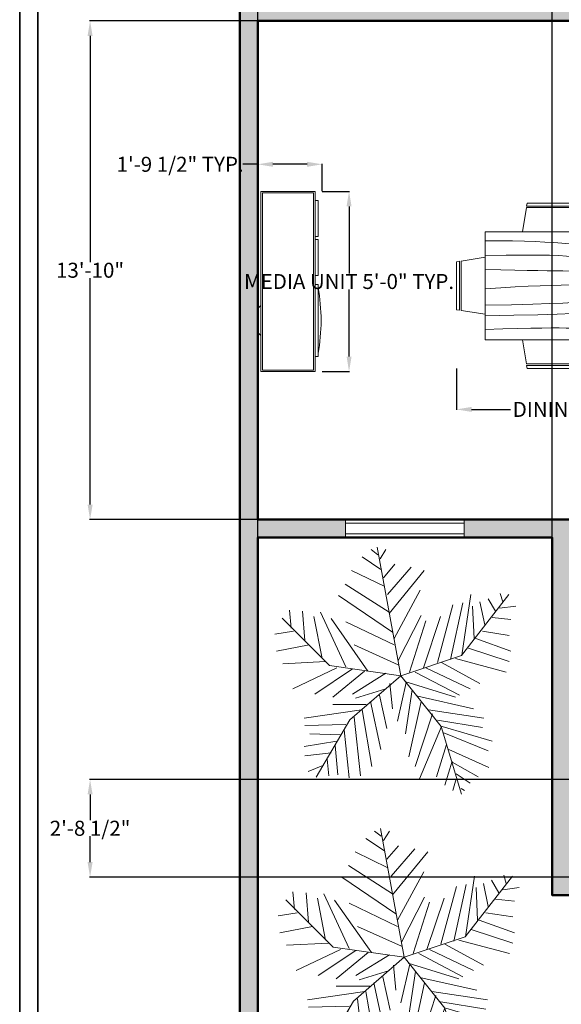
# Model space of a CAD drawing. Units: inches. Extents: x -60 to 743, y -483 to 510.
# Tile 2 of 7: x -60 to 120, y -299 to 29. Entities that reach past the tile are written whole.
import ezdxf

# ---------------------------------------------------------------- set-up
doc = ezdxf.new("R2010")
doc.units = ezdxf.units.IN
doc.header["$MEASUREMENT"] = 0
for name, color, linetype, lineweight in [('A-ANNO-DIMS', 2, 'Continuous', 18), ('A-ANNO-TTLB', 7, 'Continuous', 35), ('A-WALL-PATT', 30, 'Continuous', 13), ('FURNITURE', 40, 'Continuous', 18), ('TREES', 80, 'Continuous', 13), ('WALL BOUNDRY', 10, 'Continuous', 50), ('WINDOW', 200, 'Continuous', 18)]:
    doc.layers.add(name, color=color, linetype=linetype, lineweight=lineweight)
doc.styles.get("Standard").update_dxf_attribs({"font": 'arial.ttf'})
doc.dimstyles.get("Standard").update_dxf_attribs({"dimtxt": 5, "dimasz": 5, "dimexe": 0.18, "dimexo": 0.0625, "dimgap": 0.09, "dimtad": 0, "dimtih": 1, "dimtoh": 1, "dimdec": 1, "dimzin": 0, "dimdsep": 46, "dimlunit": 4, "dimtxsty": 'Standard', "dimcen": 0.09, "dimadec": 0, "dimazin": 0, "dimtfac": 1, "dimtdec": 1, "dimtofl": 0, "dimtmove": 0, "dimatfit": 3, "dimfxl": 1, "dimtolj": 1, "dimtzin": 0, "dimarcsym": 0})

# ---------------------------------------------------------------- blocks, each defined once
blk = doc.blocks.new('Dining Set - 36 x 72 in.')
for p, q in [((-22, 27.5), (-22.1562, 26.50042)), ((-5.8416, 26.5), (-22.1534, 26.5)), ((-22, 27.5), (-6, 27.5)), ((-5.8437, 26.49966), (-6, 27.5)), ((6, 27.5), (5.8438, 26.50042)), ((22.1584, 26.5), (5.8466, 26.5)), ((6, 27.5), (22, 27.5)), ((22.1563, 26.49966), (22, 27.5)), ((-22.2343, 26.00059), (-23.4847, 17.99762)), ((-22.2304, 26), (-5.7608, 26)), ((-4.5152, 17.99762), (-5.7655, 25.99926)), ((5.7657, 26.00059), (4.5153, 17.99762)), ((5.7696, 26), (22.2392, 26)), ((23.4848, 17.99762), (22.2345, 25.99926)), ((36, 18), (-36, 18)), ((-36, 18), (-36, -18)), ((36, -18), (36, 18)), ((-45.5, 8), (-44.5004, 8.15617)), ((-45.5, 8), (-45.5, -8)), ((-44.5, -8.15843), (-44.5, 8.15338)), ((-44.0006, 8.23428), (-35.9976, 9.48474)), ((-44, 8.23041), (-44, -8.23915)), ((44.0006, 8.23428), (35.9976, 9.48474)), ((44, 8.23041), (44, -8.23915)), ((44.5, -8.15843), (44.5, 8.15338)), ((45.5, 8), (44.5005, 8.15617)), ((45.5, 8), (45.5, -8)), ((-44.4997, -8.15631), (-45.5, -8)), ((-35.9976, -9.48476), (-43.9993, -8.2345)), ((35.9976, -9.48476), (43.9993, -8.2345)), ((44.4997, -8.15631), (45.5, -8)), ((-36, -18), (36, -18)), ((-22.2343, -26.0006), (-23.4847, -17.99762)), ((-4.5152, -17.99762), (-5.7655, -25.99928)), ((5.7657, -26.0006), (4.5153, -17.99762)), ((23.4848, -17.99762), (22.2345, -25.99928)), ((-22.2304, -26), (-5.7608, -26)), ((5.7696, -26), (22.2392, -26)), ((-22, -27.5), (-22.1562, -26.50044)), ((-5.8416, -26.5), (-22.1534, -26.5)), ((-22, -27.5), (-6, -27.5)), ((-5.8437, -26.49967), (-6, -27.5)), ((6, -27.5), (5.8438, -26.50044)), ((22.1584, -26.5), (5.8466, -26.5)), ((6, -27.5), (22, -27.5)), ((22.1563, -26.49967), (22, -27.5))]:
    blk.add_line(p, q)
for points in [[(-36, 15), (-31.1772, 14.97754), (-26.8079, 14.91406), (-22.8538, 14.81543), (-19.276, 14.6875), (-16.0362, 14.53613), (-13.0957, 14.36718), (-10.4159, 14.18652), (-7.9583, 14), (-5.6904, 13.81315), (-3.6035, 13.63021), (-1.6954, 13.45508), (0.0365, 13.29166), (1.5945, 13.14388), (2.9811, 13.01562), (4.1988, 12.9108), (5.25, 12.83333), (6.1393, 12.78613), (6.8802, 12.76823), (7.4883, 12.77767), (7.9792, 12.8125), (8.3685, 12.87077), (8.6719, 12.95052), (8.9049, 13.0498), (9.0833, 13.16666), (9.2205, 13.29899), (9.3216, 13.44401), (9.3895, 13.59879), (9.4271, 13.76041), (9.4373, 13.92594), (9.4232, 14.09245), (9.3875, 14.257), (9.3333, 14.41666), (9.2638, 14.56917), (9.1836, 14.71484), (9.0975, 14.85465), (9.0104, 14.98958), (8.9272, 15.1206), (8.8529, 15.2487), (8.7922, 15.37483), (8.75, 15.5), (8.7305, 15.62467), (8.7344, 15.74739), (8.7617, 15.86621), (8.8125, 15.97916), (8.8867, 16.08431), (8.9844, 16.17968), (9.1055, 16.26334), (9.25, 16.33333), (9.4189, 16.38802), (9.6172, 16.42708), (9.8506, 16.45052), (10.125, 16.45833), (10.4463, 16.45052), (10.8203, 16.42708), (11.2529, 16.38802), (11.75, 16.33333), (12.3184, 16.26318), (12.9694, 16.17838), (13.7151, 16.07991), (14.5677, 15.96875), (15.5395, 15.84586), (16.6426, 15.71224), (17.8893, 15.56884), (19.2917, 15.41666), (20.859, 15.25667), (22.5879, 15.08984), (24.4721, 14.91715), (26.5052, 14.73958), (28.6809, 14.5581), (30.9929, 14.3737), (33.4347, 14.18733), (36, 14)], [(-36, 10), (-28.9766, 10.14274), (-23.1725, 10.20442), (-18.4241, 10.19775), (-14.5677, 10.13541), (-11.4399, 10.03011), (-8.877, 9.89453), (-6.7154, 9.74137), (-4.7917, 9.58333), (-2.9698, 9.43082), (-1.2246, 9.28515), (0.4415, 9.14534), (2.026, 9.01041), (3.5266, 8.87939), (4.9408, 8.7513), (6.266, 8.62516), (7.5, 8.5), (8.6411, 8.37549), (9.6914, 8.2539), (10.6538, 8.13818), (11.5312, 8.03125), (12.3267, 7.93603), (13.043, 7.85547), (13.6831, 7.79248), (14.25, 7.75), (14.7471, 7.7303), (15.1797, 7.73307), (15.5537, 7.75732), (15.875, 7.80208), (16.1494, 7.86637), (16.3828, 7.94922), (16.5811, 8.04964), (16.75, 8.16666), (16.8944, 8.29915), (17.0143, 8.44531), (17.1089, 8.60319), (17.1771, 8.77083), (17.218, 8.94629), (17.2305, 9.1276), (17.2137, 9.31282), (17.1667, 9.5), (17.0895, 9.6875), (16.987, 9.875), (16.8649, 10.0625), (16.7292, 10.25), (16.5856, 10.4375), (16.4401, 10.625), (16.2985, 10.8125), (16.1667, 11), (16.05, 11.18733), (15.9518, 11.3737), (15.8752, 11.5581), (15.8229, 11.73958), (15.798, 11.91715), (15.8034, 12.08984), (15.842, 12.25667), (15.9167, 12.41666), (16.0295, 12.56836), (16.1784, 12.70833), (16.3605, 12.83268), (16.5729, 12.9375), (16.8127, 13.01888), (17.0768, 13.07291), (17.3625, 13.0957), (17.6667, 13.08333), (17.9894, 13.03312), (18.3418, 12.94726), (18.7382, 12.82918), (19.1927, 12.68229), (19.7195, 12.51001), (20.3327, 12.31575), (21.0465, 12.10294), (21.875, 11.875), (22.8357, 11.63354), (23.959, 11.37304), (25.2786, 11.08618), (26.8282, 10.76562), (28.6414, 10.40405), (30.752, 9.99414), (33.1936, 9.52856), (36, 9)], [(-36, 5.5), (-30.7157, 5.3348), (-26.069, 5.20963), (-21.9946, 5.11767), (-18.4271, 5.05208), (-15.3009, 5.00602), (-12.5508, 4.97265), (-10.1112, 4.94515), (-7.9167, 4.91666), (-5.909, 4.88167), (-4.0586, 4.83984), (-2.3429, 4.79215), (-0.7396, 4.73958), (0.7739, 4.6831), (2.22, 4.6237), (3.6213, 4.56233), (5, 4.5), (6.373, 4.43782), (7.7344, 4.3776), (9.0723, 4.32129), (10.375, 4.27083), (11.6309, 4.22819), (12.8281, 4.19531), (13.9551, 4.17415), (15, 4.16666), (15.954, 4.17448), (16.819, 4.19791), (17.6001, 4.23698), (18.3021, 4.29166), (18.9299, 4.36198), (19.4883, 4.44791), (19.9823, 4.54948), (20.4167, 4.66666), (20.7969, 4.79899), (21.1302, 4.94401), (21.4245, 5.09879), (21.6875, 5.26041), (21.9271, 5.42594), (22.1511, 5.59245), (22.3672, 5.757), (22.5834, 5.91666), (22.8065, 6.06868), (23.0404, 6.21093), (23.2879, 6.34147), (23.5521, 6.45833), (23.8358, 6.55957), (24.142, 6.64323), (24.4735, 6.70735), (24.8334, 6.75), (25.2235, 6.76969), (25.642, 6.76692), (26.0858, 6.74267), (26.5521, 6.69791), (27.0379, 6.63362), (27.5404, 6.55078), (28.0565, 6.45036), (28.5834, 6.33333), (29.1242, 6.19987), (29.7071, 6.04687), (30.3661, 5.87044), (31.1354, 5.66666), (32.0493, 5.43164), (33.142, 5.16146), (34.4475, 4.85221), (36, 4.5)], [(-36, -1), (-30.7915, -0.6591), (-26.0195, -0.38216), (-21.6519, -0.16284), (-17.6563, 0.00521), (-14.0005, 0.12833), (-10.6523, 0.21289), (-7.5796, 0.26522), (-4.75, 0.29166), (-2.134, 0.29793), (0.2878, 0.28711), (2.5317, 0.26163), (4.6146, 0.22396), (6.5529, 0.17651), (8.3633, 0.12174), (10.0623, 0.06209), (11.6667, 0), (13.1899, -0.06201), (14.6341, -0.1211), (15.9982, -0.17432), (17.2813, -0.21875), (18.4823, -0.25147), (19.6003, -0.26953), (20.6343, -0.27002), (21.5834, -0.25), (22.4481, -0.20768), (23.2357, -0.14584), (23.9549, -0.06836), (24.6146, 0.02083), (25.2235, 0.11784), (25.7904, 0.21875), (26.3241, 0.31966), (26.8334, 0.41666), (27.3265, 0.50618), (27.8099, 0.58593), (28.2894, 0.65397), (28.7709, 0.70833), (29.2601, 0.74707), (29.763, 0.76823), (30.2855, 0.76985), (30.8334, 0.75), (31.4088, 0.70784), (31.9994, 0.64713), (32.589, 0.57275), (33.1615, 0.48958), (33.7008, 0.4025), (34.1908, 0.3164), (34.6153, 0.23616), (34.9584, 0.16666), (35.2099, 0.11165), (35.3848, 0.07031), (35.504, 0.04069), (35.5886, 0.02083), (35.6594, 0.00879), (35.7377, 0.0026), (35.8442, 0.00032), (36, 0)], [(-36, -6.5), (-27.1843, -6.31267), (-20.084, -6.1263), (-14.469, -5.9419), (-10.1094, -5.76042), (-6.7752, -5.58285), (-4.2363, -5.41016), (-2.2629, -5.24333), (-0.625, -5.08334), (0.8708, -4.93099), (2.2715, -4.78646), (3.5872, -4.64974), (4.8281, -4.52084), (6.0046, -4.39974), (7.127, -4.28646), (8.2053, -4.18099), (9.25, -4.08334), (10.2705, -3.99382), (11.2734, -3.91407), (12.2647, -3.84603), (13.25, -3.79167), (14.2354, -3.75293), (15.2266, -3.73177), (16.2295, -3.73015), (17.25, -3.75), (18.2912, -3.79248), (19.3451, -3.85547), (20.4009, -3.93604), (21.4479, -4.03125), (22.4754, -4.13819), (23.4727, -4.25391), (24.4289, -4.37549), (25.3334, -4.5), (26.1785, -4.62492), (26.9694, -4.74935), (27.7145, -4.87281), (28.4219, -4.99479), (29.1, -5.11483), (29.7572, -5.23242), (30.4016, -5.34709), (31.0417, -5.45834), (31.6837, -5.56437), (32.3262, -5.65821), (32.9658, -5.73153), (33.599, -5.77604), (34.2224, -5.78345), (34.8327, -5.74545), (35.4264, -5.65373), (36, -5.5)], [(-36, -10), (-26.4022, -9.81299), (-18.4675, -9.62891), (-11.9839, -9.45069), (-6.7396, -9.28125), (-2.5226, -9.12354), (0.8789, -8.98047), (3.6769, -8.85498), (6.0833, -8.75), (8.2767, -8.66765), (10.3021, -8.60677), (12.1712, -8.56543), (13.8958, -8.54167), (15.4876, -8.53353), (16.9583, -8.53907), (18.3197, -8.55632), (19.5834, -8.58334), (20.7616, -8.61841), (21.8685, -8.66081), (22.9188, -8.71004), (23.9271, -8.76563), (24.9081, -8.82707), (25.8763, -8.89388), (26.8465, -8.96558), (27.8334, -9.04167), (28.8474, -9.12118), (29.8828, -9.20117), (30.93, -9.27824), (31.9792, -9.34896), (33.0205, -9.40991), (34.0443, -9.45768), (35.0407, -9.48885), (36, -9.5)], [(-36, -14.5), (-30.0881, -14.33513), (-25.0332, -14.21224), (-20.7312, -14.12647), (-17.0781, -14.07292), (-13.97, -14.04671), (-11.3027, -14.04297), (-8.9724, -14.05681), (-6.875, -14.08334), (-4.9224, -14.11833), (-3.0905, -14.16016), (-1.3709, -14.20785), (0.2448, -14.26042), (1.7647, -14.3169), (3.1973, -14.3763), (4.5507, -14.43767), (5.8333, -14.5), (7.0554, -14.5621), (8.235, -14.62175), (9.3922, -14.67652), (10.5469, -14.72396), (11.7192, -14.76164), (12.929, -14.78711), (14.1965, -14.79794), (15.5417, -14.79167), (16.9933, -14.76424), (18.6152, -14.70508), (20.4804, -14.60197), (22.6615, -14.44271), (25.2312, -14.21509), (28.2624, -13.9069), (31.8277, -13.50594), (36, -13)]]:
    blk.add_lwpolyline(points)
blk = doc.blocks.new('Entertainment Center')
for p, q in [((-4, 0), (-5, -1)), ((4, 0), (-4, 0)), ((5, -1), (4, 0)), ((-17, -19), (-17, -1)), ((-17, -1), (43, -1)), ((-16.5, -18.5), (-16.5, -1.5)), ((-16.5, -1.5), (42.5, -1.5)), ((42.5, -1.5), (42.5, -18.5)), ((43, -1), (43, -19)), ((43, -19), (-17, -19)), ((42.5, -18.5), (-16.5, -18.5)), ((-12, -20), (-12, -19)), ((12, -19), (12, -20)), ((15, -20), (15, -19)), ((27, -19), (27, -20)), ((28, -20), (28, -19)), ((40, -19), (40, -20)), ((12, -20), (-12, -20)), ((27, -20), (15, -20)), ((40, -20), (28, -20))]:
    blk.add_line(p, q)
blk.add_arc((0, 40), 61, 259.6111, 280.3889)
blk = doc.blocks.new('*U21')
for p, q in [((0, 0), (-266.7, 1447.8)), ((-221.9198, 1197.3052), (-433.5526, 1338.8594)), ((-258.7244, 1362.456), (-332.3336, 1421.4348)), ((-231.1146, 1315.2628), (-166.7002, 1421.4348)), ((-194.31, 1102.9442), (-65.4812, 1256.284)), ((-148.3106, 914.1968), (118.5418, 1220.9018)), ((-185.1152, 1008.5578), (-553.1612, 1185.4942)), ((-129.8956, 701.8528), (265.7602, 1185.4942)), ((-129.8956, 713.6638), (-626.7704, 1032.1544)), ((-93.091, 489.5342), (-700.3796, 902.3858)), ((-74.7014, 418.7444), (219.7608, 961.39)), ((685.8, 228.6), (1219.2, 914.4)), ((689.0258, 230.0224), (790.2448, 914.1968)), ((1121.4862, 925.9824), (1149.0706, 831.6214)), ((412.9786, 147.447), (587.8068, 796.2392)), ((560.197, 182.8292), (698.2206, 819.8358)), ((808.6344, 784.4282), (827.0494, 418.7444)), ((891.4384, 831.6214), (946.658, 572.1096)), ((983.4626, 867.0036), (1066.2666, 725.4494)), ((1112.2914, 760.8316), (1296.3144, 784.4282)), ((-1234.059, 536.7274), (-1252.4486, 737.2604)), ((-1105.2302, 725.4494), (-1077.6458, 395.1732)), ((-976.4268, 666.4706), (-884.4026, 194.6402)), ((-902.8176, 713.6638), (-617.5756, 100.2538)), ((-28.6766, 171.0436), (228.9556, 678.2816)), ((256.5654, 88.4682), (449.7832, 666.4706)), ((-800.1, 114.3), (-1333.5, 647.7)), ((-369.1382, 53.086), (-783.1836, 642.874)), ((-617.5756, 607.4918), (-74.7014, 347.98)), ((100.1268, 41.275), (284.1498, 619.2774)), ((1029.462, 654.685), (1241.0948, 631.0884)), ((-1206.4492, 501.3198), (-1418.082, 465.9376)), ((919.0482, 501.3198), (1222.6798, 454.152)), ((-1031.621, 347.98), (-1399.667, 277.1902)), ((-525.5514, 347.98), (-28.6766, 123.8504)), ((845.439, 418.7444), (1241.0948, 277.1902)), ((0, 0), (685.8, 228.6)), ((753.4148, 312.5978), (1222.6798, 159.2326)), ((-847.598, 159.2326), (-1326.0578, 135.636)), ((0, 0), (-800.1, 114.3)), ((458.978, 147.447), (891.4384, -88.4682)), ((615.4166, 194.6402), (1185.8752, 41.275)), ((-718.7946, 88.4682), (-1215.644, -147.447)), ((-543.9664, 76.6572), (-967.2066, -206.4512)), ((-405.9428, 53.086), (-764.794, -241.8334)), ((0, 0), (-571.5, -495.3)), ((-166.7002, 29.4894), (-543.9664, -206.4512)), ((0, 0), (457.2, -571.5)), ((164.5412, 41.275), (661.416, -218.2368)), ((284.1498, 88.4682), (781.0246, -147.447)), ((-120.7008, -88.4682), (-93.091, -371.5766)), ((63.3222, -76.6826), (-37.8714, -513.1308)), ((44.9326, -64.897), (615.4166, -241.8334)), ((-166.7002, -147.447), (-507.1618, -253.619)), ((-240.3094, -218.2368), (-157.5054, -595.7062)), ((127.7366, -159.258), (54.1274, -654.685)), ((-387.5278, -324.4088), (-764.794, -324.4088)), ((-341.5284, -289.0012), (-221.9198, -831.6214)), ((228.9556, -289.0012), (90.932, -914.1968)), ((192.151, -230.0224), (817.8292, -371.5766)), ((-442.7474, -383.3876), (-1086.8406, -477.7486)), ((-433.5526, -383.3876), (-323.1134, -1020.3688)), ((357.759, -430.5554), (164.5412, -1020.3688)), ((311.7596, -383.3876), (937.4378, -477.7486)), ((-617.5756, -548.5384), (-1077.6458, -560.324)), ((-571.5, -495.3), (-952.5, -1143)), ((-525.5514, -465.963), (-451.9422, -1126.5408)), ((412.9786, -501.3452), (919.0482, -583.9206)), ((-681.9646, -666.496), (-1022.4262, -654.685)), ((-635.9652, -607.5172), (-580.771, -1150.1374)), ((458.978, -572.1096), (210.5406, -1161.923)), ((457.2, -571.5), (685.8, -1333.5)), ((468.1982, -572.1096), (1029.462, -737.2604)), ((486.5878, -642.8994), (983.4626, -843.4324)), ((-718.7946, -737.2604), (-1086.8406, -796.2392)), ((514.1976, -772.6426), (403.7838, -1138.3264)), ((-783.1836, -867.029), (-1077.6458, -902.4112)), ((-737.1842, -784.4536), (-709.5744, -1114.7298)), ((541.8074, -831.6214), (992.6574, -1032.1544)), ((-829.2084, -937.7934), (-810.7934, -1126.5408)), ((578.612, -961.39), (495.7826, -1232.7128)), ((578.612, -973.1756), (873.0488, -1138.3264)), ((-875.2078, -1008.5832), (-1040.8412, -1079.3476)), ((624.6114, -1102.9442), (781.0246, -1209.1162)), ((624.6114, -1161.923), (587.8068, -1291.6916)), ((679.8056, -1268.095), (716.6102, -1291.6916))]:
    blk.add_line(p, q)
blk = doc.blocks.new('*D36')
at = {"layer": 'A-ANNO-DIMS', "color": 0, "lineweight": -2, "transparency": 16777216}
for p, q in [((40.54, -28.32), (49.66, -28.32)), ((49.48, -33.32), (49.48, -55.67)), ((49.48, -83.32), (49.48, -60.96)), ((40.54, -88.32), (49.66, -88.32))]:
    blk.add_line(p, q, dxfattribs=at)
at = {"layer": 'A-ANNO-DIMS', "color": 0, "transparency": 16777216}
for points in [[(48.65, -33.32), (50.31, -33.32), (49.48, -28.32)], [(48.65, -83.32), (50.31, -83.32), (49.48, -88.32)]]:
    blk.add_solid(points, dxfattribs=at)
at = {"layer": 'Defpoints', "color": 0, "transparency": 16777216}
for p in [(40.48, -28.32), (49.48, -28.32), (40.48, -88.32)]:
    blk.add_point(p, dxfattribs=at)
at = {"layer": 'A-ANNO-DIMS', "color": 0, "transparency": 16777216, "insert": (49.48, -58.32), "char_height": 5, "attachment_point": 5}
blk.add_mtext('\\A1;MEDIA UNIT 5\'-0" TYP.', dxfattribs=at)
blk = doc.blocks.new('*D37')
at = {"layer": 'A-ANNO-DIMS', "color": 0, "lineweight": -2, "transparency": 16777216}
for p, q in [((19.15, -19.32), (14.15, -19.32)), ((19.15, -28.25), (19.15, -19.14)), ((35.48, -19.32), (24.15, -19.32)), ((40.48, -28.25), (40.48, -19.14))]:
    blk.add_line(p, q, dxfattribs=at)
at = {"layer": 'A-ANNO-DIMS', "color": 0, "transparency": 16777216}
for points in [[(24.15, -18.48), (24.15, -20.15), (19.15, -19.32)], [(35.48, -18.48), (35.48, -20.15), (40.48, -19.32)]]:
    blk.add_solid(points, dxfattribs=at)
at = {"layer": 'Defpoints', "color": 0, "transparency": 16777216}
for p in [(19.15, -19.32), (19.15, -28.32), (40.48, -28.32)]:
    blk.add_point(p, dxfattribs=at)
at = {"layer": 'A-ANNO-DIMS', "color": 0, "transparency": 16777216, "insert": (-6.77, -19.32), "char_height": 5, "attachment_point": 5}
blk.add_mtext('\\A1;1\'-9 1/2" TYP.', dxfattribs=at)
blk = doc.blocks.new('*D62')
at = {"layer": 'A-ANNO-DIMS', "color": 0, "lineweight": -2, "transparency": 16777216}
for p, q in [((85.25, -87.32), (85.25, -101.08)), ((176.25, -87.32), (176.25, -101.08)), ((90.25, -100.9), (103.18, -100.9)), ((171.25, -100.9), (158.32, -100.9))]:
    blk.add_line(p, q, dxfattribs=at)
at = {"layer": 'A-ANNO-DIMS', "color": 0, "transparency": 16777216}
for points in [[(90.25, -100.07), (90.25, -101.74), (85.25, -100.9)], [(171.25, -100.07), (171.25, -101.74), (176.25, -100.9)]]:
    blk.add_solid(points, dxfattribs=at)
at = {"layer": 'Defpoints', "color": 0, "transparency": 16777216}
for p in [(85.25, -87.25), (176.25, -87.25), (176.25, -100.9)]:
    blk.add_point(p, dxfattribs=at)
at = {"layer": 'A-ANNO-DIMS', "color": 0, "transparency": 16777216, "insert": (130.75, -100.9), "char_height": 5, "attachment_point": 5}
blk.add_mtext('\\A1;DINING SET 7\'-7"', dxfattribs=at)
blk = doc.blocks.new('*D72')
at = {"layer": 'A-ANNO-DIMS', "color": 0, "lineweight": -2, "transparency": 16777216}
for p, q in [((19.08, 28.42), (-36.93, 28.42)), ((-36.75, 23.42), (-36.75, -51.93)), ((-36.75, -132.58), (-36.75, -57.22)), ((19.08, -137.58), (-36.93, -137.58))]:
    blk.add_line(p, q, dxfattribs=at)
at = {"layer": 'A-ANNO-DIMS', "color": 0, "transparency": 16777216}
for points in [[(-37.58, 23.42), (-35.91, 23.42), (-36.75, 28.42)], [(-37.58, -132.58), (-35.91, -132.58), (-36.75, -137.58)]]:
    blk.add_solid(points, dxfattribs=at)
at = {"layer": 'Defpoints', "color": 0, "transparency": 16777216}
for p in [(19.15, 28.42), (-36.75, -137.58), (19.15, -137.58)]:
    blk.add_point(p, dxfattribs=at)
at = {"layer": 'A-ANNO-DIMS', "color": 0, "transparency": 16777216, "insert": (-36.75, -54.58), "char_height": 5, "attachment_point": 5}
blk.add_mtext('\\A1;13\'-10"', dxfattribs=at)
blk = doc.blocks.new('*D73')
at = {"layer": 'A-ANNO-DIMS', "color": 0, "lineweight": -2, "transparency": 16777216}
for p, q in [((19.15, -143.52), (19.15, 465.7)), ((24.15, 465.52), (61.41, 465.52)), ((112.15, 465.52), (74.89, 465.52)), ((117.15, -143.52), (117.15, 465.7))]:
    blk.add_line(p, q, dxfattribs=at)
at = {"layer": 'A-ANNO-DIMS', "color": 0, "transparency": 16777216}
for points in [[(24.15, 466.36), (24.15, 464.69), (19.15, 465.52)], [(112.15, 466.36), (112.15, 464.69), (117.15, 465.52)]]:
    blk.add_solid(points, dxfattribs=at)
at = {"layer": 'Defpoints', "color": 0, "transparency": 16777216}
for p in [(117.15, 465.52), (19.15, -143.58), (117.15, -143.58)]:
    blk.add_point(p, dxfattribs=at)
at = {"layer": 'A-ANNO-DIMS', "color": 0, "transparency": 16777216, "insert": (68.15, 465.52), "char_height": 5, "attachment_point": 5}
blk.add_mtext('\\A1;8\'-2"', dxfattribs=at)
blk = doc.blocks.new('*D77')
at = {"layer": 'A-ANNO-DIMS', "color": 0, "lineweight": -2, "transparency": 16777216}
for p, q in [((154.93, -224.05), (-36.93, -224.05)), ((-36.75, -229.05), (-36.75, -237.64)), ((-36.75, -251.58), (-36.75, -242.99)), ((123.08, -256.58), (-36.93, -256.58))]:
    blk.add_line(p, q, dxfattribs=at)
at = {"layer": 'A-ANNO-DIMS', "color": 0, "transparency": 16777216}
for points in [[(-37.58, -229.05), (-35.91, -229.05), (-36.75, -224.05)], [(-37.58, -251.58), (-35.91, -251.58), (-36.75, -256.58)]]:
    blk.add_solid(points, dxfattribs=at)
at = {"layer": 'Defpoints', "color": 0, "transparency": 16777216}
for p in [(154.99, -224.05), (-36.75, -256.58), (123.15, -256.58)]:
    blk.add_point(p, dxfattribs=at)
at = {"layer": 'A-ANNO-DIMS', "color": 0, "transparency": 16777216, "insert": (-36.75, -240.31), "char_height": 5, "attachment_point": 5}
blk.add_mtext('\\A1;2\'-8 1/2"', dxfattribs=at)

msp = doc.modelspace()

# ---------------------------------------------------------------- hatches: boundary and pattern name
at = {"layer": 'A-WALL-PATT'}
h = msp.add_hatch(color=256, dxfattribs=at)
h.dxf.hatch_style = 1
h.paths.add_polyline_path([(412.35, 168.77), (415.89, 168.77), (415.89, 114.92), (412.35, 114.92)], flags=16)
h.paths.add_polyline_path([(87.81, -138.81), (87.81, -142.35), (48.31, -142.32), (48.31, -138.78)], flags=16)
h.paths.add_polyline_path([(459.53, -138.78), (513.39, -138.78), (513.39, -142.32), (459.53, -142.32)], flags=16)
h.paths.add_polyline_path([(164.84, -257.78), (218.7, -257.78), (218.7, -261.32), (164.84, -261.32)], flags=16)
h.paths.add_polyline_path([(417.15, 114.92), (415.89, 114.92), (415.89, 168.77), (417.15, 168.77), (417.15, 195.42), (411.15, 195.42), (411.15, 168.77), (412.35, 168.77), (412.35, 114.92), (411.15, 114.92), (411.15, 28.42), (610.15, 28.42), (610.15, -43.58), (508.15, -43.58), (508.15, -49.58), (610.15, -49.58), (610.15, -137.58), (513.39, -137.58), (513.39, -138.78), (459.53, -138.78), (459.53, -137.58), (359.15, -137.58), (359.15, -143.58), (377.15, -143.58), (377.15, -292.58), (383.15, -292.58), (383.15, -143.58), (459.53, -143.58), (459.53, -142.32), (513.39, -142.32), (513.39, -143.58), (610.15, -143.58), (610.15, -415.58), (610.15, -421.58), (616.15, -421.58), (616.15, 418.42), (13.15, 418.42), (13.15, -421.58), (19.15, -421.58), (430.15, -421.58), (430.15, -415.58), (19.15, -415.58), (19.15, -143.58), (48.31, -143.58), (48.31, -142.32), (87.81, -142.35), (87.81, -143.58), (117.15, -143.58), (117.15, -262.58), (164.84, -262.58), (164.84, -261.32), (218.7, -261.32), (218.7, -262.58), (273.15, -262.58), (273.15, -292.58), (279.15, -292.58), (279.15, -143.58), (297.15, -143.58), (297.15, -137.58), (273.15, -137.58), (273.15, -256.58), (218.7, -256.58), (218.7, -257.78), (164.84, -257.78), (164.84, -256.58), (123.15, -256.58), (123.15, -143.58), (225.15, -143.58), (225.15, -137.58), (87.81, -137.58), (87.81, -138.81), (48.31, -138.78), (48.31, -137.58), (19.15, -137.58), (19.15, 28.42), (187.15, 28.42), (187.15, 34.42), (19.15, 34.42), (19.15, 178.42), (273.15, 178.42), (273.15, 184.42), (19.15, 184.42), (19.15, 345.58), (195.14, 345.58), (195.14, 348.9), (19.15, 348.9), (19.15, 412.42), (267.15, 412.42), (267.15, 319.83), (273.15, 319.83), (273.15, 412.42), (411.15, 412.42), (411.15, 376.24), (417.15, 376.24), (417.15, 412.42), (610.15, 412.42), (610.15, 249.42), (411.15, 249.42), (411.15, 243.42), (610.15, 243.42), (610.15, 34.42), (417.15, 34.42)])
h = msp.add_hatch(color=256, dxfattribs=at)
h.dxf.hatch_style = 1
h.paths.add_polyline_path([(273.15, 265.98), (267.15, 265.98), (267.15, 232.42), (273.15, 232.42)])
h.paths.add_polyline_path([(417.15, 322.39), (411.15, 322.39), (411.15, 297.42), (417.15, 297.42)])
h.paths.add_polyline_path([(417.15, 195.42), (411.15, 195.42), (411.15, 168.77), (417.15, 168.77)])
h.paths.add_polyline_path([(459.53, -137.58), (359.15, -137.58), (359.15, -143.58), (377.15, -143.58), (377.15, -292.58), (383.15, -292.58), (383.15, -143.58), (459.53, -143.58)])
h.paths.add_polyline_path([(279.15, -143.58), (297.15, -143.58), (297.15, -137.58), (273.15, -137.58), (273.15, -256.58), (218.7, -256.58), (218.7, -262.58), (273.15, -262.58), (273.15, -292.58), (279.15, -292.58)])
h.paths.add_polyline_path([(123.15, -143.58), (225.15, -143.58), (225.15, -137.58), (87.81, -137.58), (87.81, -143.58), (117.15, -143.58), (117.15, -262.58), (164.84, -262.58), (164.84, -256.58), (123.15, -256.58)])
h = msp.add_hatch(color=256, dxfattribs=at)
h.dxf.hatch_style = 1
h.paths.add_polyline_path([(48.31, -138.78), (87.81, -138.81), (87.81, -142.35), (48.31, -142.32)], flags=17)
h.paths.add_polyline_path([(164.84, -257.78), (218.7, -257.78), (218.7, -261.32), (164.84, -261.32)], flags=17)
h.paths.add_polyline_path([(48.31, -142.32), (87.81, -142.35), (87.81, -138.81), (48.31, -138.78)])
h.paths.add_polyline_path([(164.84, -261.32), (218.7, -261.32), (218.7, -257.78), (164.84, -257.78)])

# ---------------------------------------------------------------- linework, layer by layer
at = {"layer": 'A-ANNO-TTLB'}
for points in [[(742.84, -483.31), (-60.19, -483.31), (-60.19, 510.12), (742.84, 510.12)], [(736.84, -477.31), (-54.19, -477.31), (-54.19, 504.12), (736.84, 504.12)]]:
    msp.add_lwpolyline(points, close=True, dxfattribs=at)
at = {"layer": 'WALL BOUNDRY'}
msp.add_lwpolyline([(610.15, -415.58), (610.15, -421.58), (616.15, -421.58), (616.15, 418.42), (13.15, 418.42), (13.15, -421.58), (19.15, -421.58), (430.15, -421.58), (430.15, -415.58), (19.15, -415.58), (19.15, -143.58), (117.15, -143.58), (117.15, -262.58), (273.15, -262.58), (273.15, -292.58), (279.15, -292.58), (377.15, -292.58), (383.15, -292.58), (383.15, -143.58), (610.15, -143.58)], close=True, dxfattribs=at)
msp.add_lwpolyline([(610.15, -137.58), (359.15, -137.58), (359.15, -143.58), (377.15, -143.58), (377.15, -298.27), (279.15, -298.27), (279.15, -143.58), (297.15, -143.58), (297.15, -137.58), (273.15, -137.58), (273.15, -256.58), (123.15, -256.58), (123.15, -143.58), (225.15, -143.58), (225.15, -137.58), (19.15, -137.58), (19.15, 28.42), (187.15, 28.42), (187.15, 34.42)], dxfattribs=at)
at = {"layer": 'WINDOW'}
for points in [[(87.81, -137.58), (87.81, -143.58), (48.31, -143.58), (48.31, -137.58)], [(87.81, -138.81), (87.81, -142.35), (48.31, -142.32), (48.31, -138.78)]]:
    msp.add_lwpolyline(points, close=True, dxfattribs=at)

# ---------------------------------------------------------------- block references
at = {"layer": 'FURNITURE', "rotation": 89.99999999999999}
msp.add_blockref('Entertainment Center', (19.15, -71.32), dxfattribs=at)
at = {"layer": 'FURNITURE'}
msp.add_blockref('Dining Set - 36 x 72 in.', (130.75, -59.75), dxfattribs=at)
at = {"layer": 'TREES', "xscale": 0.0295751403229488, "yscale": 0.0295751403229488, "zscale": 0.0295751403229488}
for p in [(66.67, -189.54), (67.83, -283.26)]:
    msp.add_blockref('*U21', p, dxfattribs=at)

# ---------------------------------------------------------------- dimensions: what is measured, and where the dimension line sits
at = {"layer": 'A-ANNO-DIMS'}
dim = msp.add_linear_dim(base=(117.15, 465.52), p1=(19.15, -143.58), p2=(117.15, -143.58), dimstyle='Standard', override={"dimdec": 1, "dimlfac": 1, "dimrnd": 0, "dimzin": 1, "dimdsep": 46, "dimlunit": 4, "dimfrac": 2}, dxfattribs=at)
dim.commit()
dim.dimension.update_dxf_attribs({"geometry": '*D73', "text_midpoint": (68.15, 465.52)})
for base, p1, p2, picture, middle in [((-36.75, -137.58), (19.15, 28.42), (19.15, -137.58), '*D72', (-36.75, -54.58)), ((-36.75, -256.58), (154.99, -224.05), (123.15, -256.58), '*D77', (-36.75, -240.31))]:
    dim = msp.add_linear_dim(base=base, p1=p1, p2=p2, angle=90, dimstyle='Standard', override={"dimdec": 1, "dimlfac": 1, "dimrnd": 0, "dimzin": 1, "dimdsep": 46, "dimlunit": 4, "dimfrac": 2}, dxfattribs=at)
    dim.commit()
    dim.dimension.update_dxf_attribs({"geometry": picture, "text_midpoint": middle})
for base, p1, p2, angle, text, picture, middle in [((19.15, -19.32), (40.48, -28.32), (19.15, -28.32), 180, '<> TYP.', '*D37', (-6.77, -19.32)), ((49.48, -28.32), (40.48, -88.32), (40.48, -28.32), 90, 'MEDIA UNIT <> TYP.', '*D36', (49.48, -58.32))]:
    dim = msp.add_linear_dim(base=base, p1=p1, p2=p2, angle=angle, text=text, dimstyle='Standard', override={"dimdec": 1, "dimlfac": 1, "dimrnd": 0, "dimzin": 1, "dimdsep": 46, "dimlunit": 4, "dimfrac": 2}, dxfattribs=at)
    dim.commit()
    dim.dimension.update_dxf_attribs({"geometry": picture, "text_midpoint": middle})
dim = msp.add_linear_dim(base=(176.25, -100.9), p1=(85.25, -87.25), p2=(176.25, -87.25), text='DINING SET <>', dimstyle='Standard', override={"dimdec": 1, "dimlfac": 1, "dimrnd": 0, "dimzin": 1, "dimdsep": 46, "dimlunit": 4, "dimfrac": 2}, dxfattribs=at)
dim.commit()
dim.dimension.update_dxf_attribs({"geometry": '*D62', "text_midpoint": (130.75, -100.9)})

doc.saveas('drawing.dxf')
